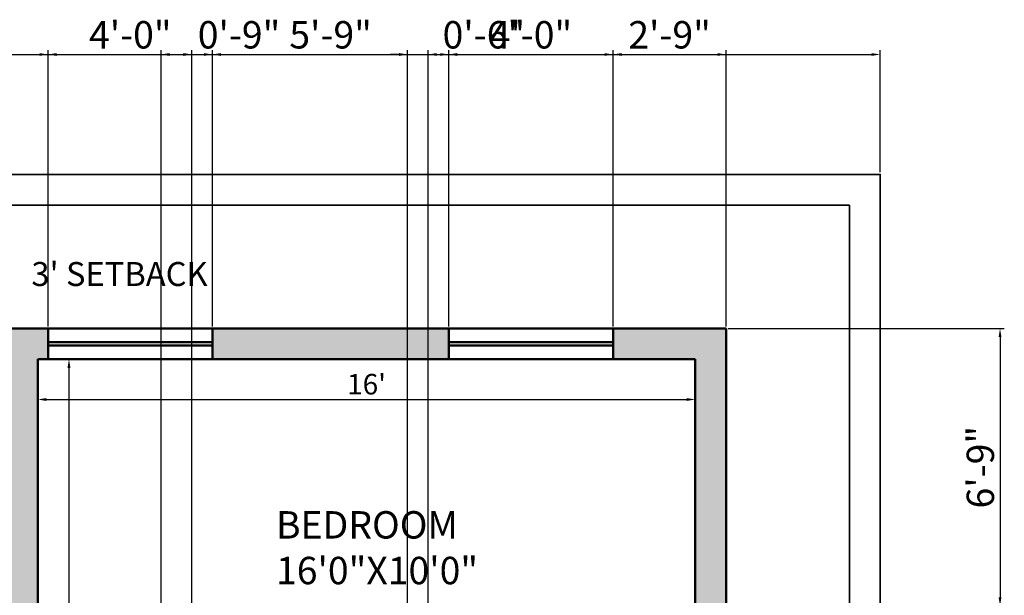
# Model space of a CAD drawing. Units: inches. Extents: x 2442 to 3851, y 589 to 2836.
# Tile 22 of 22: x 3558 to 3845, y 2668 to 2836. Entities that reach past the tile are written whole.
import ezdxf

# ---------------------------------------------------------------- set-up
doc = ezdxf.new("R2010")
doc.units = ezdxf.units.IN
for name, color, linetype, lineweight in [('A-ANNO-DIMS', 2, 'Continuous', 18), ('A-ANNO-TEXT', 7, 'Continuous', 18), ('A-AREA-IDEN', 7, 'Continuous', 18), ('A-WALL', 7, 'Continuous', 50), ('A-WALL-PATT', 8, 'Continuous', 13), ('C-PROP', 7, 'Continuous', 35)]:
    doc.layers.add(name, color=color, linetype=linetype, lineweight=lineweight)
doc.styles.get("Standard").update_dxf_attribs({"font": 'arial.ttf'})
doc.dimstyles.new('ISO-25', dxfattribs={"dimtxt": 8, "dimasz": 2.5, "dimexe": 1.25, "dimexo": 0.625, "dimtad": 1, "dimlunit": 3, "dimtxsty": 'Standard', "dimcen": 2.5, "dimadec": 0, "dimazin": 0, "dimtfac": 1, "dimtmove": 0, "dimatfit": 3, "dimfxl": 1, "dimarcsym": 0})

# ---------------------------------------------------------------- blocks, each defined once
blk = doc.blocks.new('*D116')
at = {"layer": 'A-ANNO-DIMS', "color": 0, "lineweight": -2, "transparency": 16777216}
for p, q in [((3563.02, 2736.58), (3563.02, 2724.22)), ((3755.02, 2736.58), (3755.02, 2724.22)), ((3565.52, 2725.47), (3752.52, 2725.47))]:
    blk.add_line(p, q, dxfattribs=at)
at = {"layer": 'A-ANNO-DIMS', "color": 0, "transparency": 16777216}
for points in [[(3565.52, 2725.89), (3565.52, 2725.05), (3563.02, 2725.47)], [(3752.52, 2725.89), (3752.52, 2725.05), (3755.02, 2725.47)]]:
    blk.add_solid(points, dxfattribs=at)
at = {"layer": 'Defpoints', "color": 0, "transparency": 16777216}
for p in [(3563.02, 2737.21), (3755.02, 2737.21), (3755.02, 2725.47)]:
    blk.add_point(p, dxfattribs=at)
at = {"layer": 'A-ANNO-DIMS', "color": 0, "transparency": 16777216, "insert": (3659.02, 2729.16), "char_height": 6, "attachment_point": 5}
blk.add_mtext("16'", dxfattribs=at)
blk = doc.blocks.new('*D117')
at = {"layer": 'A-ANNO-DIMS', "color": 0, "lineweight": -2, "transparency": 16777216}
for p, q in [((3563.65, 2737.21), (3573.36, 2737.21)), ((3572.11, 2734.71), (3572.11, 2565.71)), ((3563.65, 2563.21), (3573.36, 2563.21))]:
    blk.add_line(p, q, dxfattribs=at)
at = {"layer": 'A-ANNO-DIMS', "color": 0, "transparency": 16777216}
for points in [[(3571.69, 2734.71), (3572.53, 2734.71), (3572.11, 2737.21)], [(3571.69, 2565.71), (3572.53, 2565.71), (3572.11, 2563.21)]]:
    blk.add_solid(points, dxfattribs=at)
at = {"layer": 'Defpoints', "color": 0, "transparency": 16777216}
for p in [(3563.02, 2737.21), (3563.02, 2563.21), (3572.11, 2563.21)]:
    blk.add_point(p, dxfattribs=at)
at = {"layer": 'A-ANNO-DIMS', "color": 0, "transparency": 16777216, "insert": (3568.42, 2650.21), "char_height": 6, "attachment_point": 5, "rotation": 90}
blk.add_mtext('14\'-6"', dxfattribs=at)
blk = doc.blocks.new('*D218')
at = {"layer": 'A-ANNO-DIMS', "color": 0, "lineweight": -2, "transparency": 16777216}
for p, q in [((3209.02, 2791.83), (3209.02, 2827.46)), ((3809.02, 2791.83), (3809.02, 2827.46)), ((3211.52, 2826.21), (3806.52, 2826.21))]:
    blk.add_line(p, q, dxfattribs=at)
at = {"layer": 'A-ANNO-DIMS', "color": 0, "transparency": 16777216}
for points in [[(3211.52, 2826.62), (3211.52, 2825.79), (3209.02, 2826.21)], [(3806.52, 2826.62), (3806.52, 2825.79), (3809.02, 2826.21)]]:
    blk.add_solid(points, dxfattribs=at)
at = {"layer": 'Defpoints', "color": 0, "transparency": 16777216}
for p in [(3809.02, 2826.21), (3209.02, 2791.21), (3809.02, 2791.21)]:
    blk.add_point(p, dxfattribs=at)
at = {"layer": 'A-ANNO-DIMS', "color": 0, "transparency": 16777216, "insert": (3509.02, 2830.92), "char_height": 8, "attachment_point": 5}
blk.add_mtext('50\'-0"', dxfattribs=at)
blk = doc.blocks.new('*D222')
at = {"layer": 'A-ANNO-DIMS', "color": 0, "lineweight": -2, "transparency": 16777216}
for p, q in [((3512.02, 2746.83), (3512.02, 2827.46)), ((3566.02, 2746.83), (3566.02, 2827.46)), ((3514.52, 2826.21), (3563.52, 2826.21))]:
    blk.add_line(p, q, dxfattribs=at)
at = {"layer": 'A-ANNO-DIMS', "color": 0, "transparency": 16777216}
for points in [[(3514.52, 2826.62), (3514.52, 2825.79), (3512.02, 2826.21)], [(3563.52, 2826.62), (3563.52, 2825.79), (3566.02, 2826.21)]]:
    blk.add_solid(points, dxfattribs=at)
at = {"layer": 'Defpoints', "color": 0, "transparency": 16777216}
for p in [(3566.02, 2826.21), (3512.02, 2746.21), (3566.02, 2746.21)]:
    blk.add_point(p, dxfattribs=at)
at = {"layer": 'A-ANNO-DIMS', "color": 0, "transparency": 16777216, "insert": (3539.02, 2830.92), "char_height": 8, "attachment_point": 5}
blk.add_mtext('4\'-6"', dxfattribs=at)
blk = doc.blocks.new('*D223')
at = {"layer": 'A-ANNO-DIMS', "color": 0, "lineweight": -2, "transparency": 16777216}
for p, q in [((3566.02, 2746.83), (3566.02, 2827.46)), ((3614.02, 2746.83), (3614.02, 2827.46)), ((3568.52, 2826.21), (3611.52, 2826.21))]:
    blk.add_line(p, q, dxfattribs=at)
at = {"layer": 'A-ANNO-DIMS', "color": 0, "transparency": 16777216}
for points in [[(3568.52, 2826.62), (3568.52, 2825.79), (3566.02, 2826.21)], [(3611.52, 2826.62), (3611.52, 2825.79), (3614.02, 2826.21)]]:
    blk.add_solid(points, dxfattribs=at)
at = {"layer": 'Defpoints', "color": 0, "transparency": 16777216}
for p in [(3614.02, 2826.21), (3566.02, 2746.21), (3614.02, 2746.21)]:
    blk.add_point(p, dxfattribs=at)
at = {"layer": 'A-ANNO-DIMS', "color": 0, "transparency": 16777216, "insert": (3590.02, 2830.92), "char_height": 8, "attachment_point": 5}
blk.add_mtext('4\'-0"', dxfattribs=at)
blk = doc.blocks.new('*D224')
at = {"layer": 'A-ANNO-DIMS', "color": 0, "lineweight": -2, "transparency": 16777216}
for p, q in [((3614.02, 2746.83), (3614.02, 2827.46)), ((3683.02, 2746.83), (3683.02, 2827.46)), ((3616.52, 2826.21), (3680.52, 2826.21))]:
    blk.add_line(p, q, dxfattribs=at)
at = {"layer": 'A-ANNO-DIMS', "color": 0, "transparency": 16777216}
for points in [[(3616.52, 2826.62), (3616.52, 2825.79), (3614.02, 2826.21)], [(3680.52, 2826.62), (3680.52, 2825.79), (3683.02, 2826.21)]]:
    blk.add_solid(points, dxfattribs=at)
at = {"layer": 'Defpoints', "color": 0, "transparency": 16777216}
for p in [(3683.02, 2826.21), (3614.02, 2746.21), (3683.02, 2746.21)]:
    blk.add_point(p, dxfattribs=at)
at = {"layer": 'A-ANNO-DIMS', "color": 0, "transparency": 16777216, "insert": (3648.52, 2830.92), "char_height": 8, "attachment_point": 5}
blk.add_mtext('5\'-9"', dxfattribs=at)
blk = doc.blocks.new('*D225')
at = {"layer": 'A-ANNO-DIMS', "color": 0, "lineweight": -2, "transparency": 16777216}
for p, q in [((3683.02, 2746.83), (3683.02, 2827.46)), ((3731.02, 2746.83), (3731.02, 2827.46)), ((3685.52, 2826.21), (3728.52, 2826.21))]:
    blk.add_line(p, q, dxfattribs=at)
at = {"layer": 'A-ANNO-DIMS', "color": 0, "transparency": 16777216}
for points in [[(3685.52, 2826.62), (3685.52, 2825.79), (3683.02, 2826.21)], [(3728.52, 2826.62), (3728.52, 2825.79), (3731.02, 2826.21)]]:
    blk.add_solid(points, dxfattribs=at)
at = {"layer": 'Defpoints', "color": 0, "transparency": 16777216}
for p in [(3731.02, 2826.21), (3683.02, 2746.21), (3731.02, 2746.21)]:
    blk.add_point(p, dxfattribs=at)
at = {"layer": 'A-ANNO-DIMS', "color": 0, "transparency": 16777216, "insert": (3707.02, 2830.92), "char_height": 8, "attachment_point": 5}
blk.add_mtext('4\'-0"', dxfattribs=at)
blk = doc.blocks.new('*D226')
at = {"layer": 'A-ANNO-DIMS', "color": 0, "lineweight": -2, "transparency": 16777216}
for p, q in [((3731.02, 2746.83), (3731.02, 2827.46)), ((3764.02, 2746.83), (3764.02, 2827.46)), ((3733.52, 2826.21), (3761.52, 2826.21))]:
    blk.add_line(p, q, dxfattribs=at)
at = {"layer": 'A-ANNO-DIMS', "color": 0, "transparency": 16777216}
for points in [[(3733.52, 2826.62), (3733.52, 2825.79), (3731.02, 2826.21)], [(3761.52, 2826.62), (3761.52, 2825.79), (3764.02, 2826.21)]]:
    blk.add_solid(points, dxfattribs=at)
at = {"layer": 'Defpoints', "color": 0, "transparency": 16777216}
for p in [(3764.02, 2826.21), (3731.02, 2746.21), (3764.02, 2746.21)]:
    blk.add_point(p, dxfattribs=at)
at = {"layer": 'A-ANNO-DIMS', "color": 0, "transparency": 16777216, "insert": (3747.52, 2830.92), "char_height": 8, "attachment_point": 5}
blk.add_mtext('2\'-9"', dxfattribs=at)
blk = doc.blocks.new('*D227')
at = {"layer": 'A-ANNO-DIMS', "color": 0, "lineweight": -2, "transparency": 16777216}
for p, q in [((3764.65, 2746.21), (3845.27, 2746.21)), ((3844.02, 2743.71), (3844.02, 2667.71)), ((3764.65, 2665.21), (3845.27, 2665.21))]:
    blk.add_line(p, q, dxfattribs=at)
at = {"layer": 'A-ANNO-DIMS', "color": 0, "transparency": 16777216}
for points in [[(3843.61, 2743.71), (3844.44, 2743.71), (3844.02, 2746.21)], [(3843.61, 2667.71), (3844.44, 2667.71), (3844.02, 2665.21)]]:
    blk.add_solid(points, dxfattribs=at)
at = {"layer": 'Defpoints', "color": 0, "transparency": 16777216}
for p in [(3764.02, 2746.21), (3764.02, 2665.21), (3844.02, 2665.21)]:
    blk.add_point(p, dxfattribs=at)
at = {"layer": 'A-ANNO-DIMS', "color": 0, "transparency": 16777216, "insert": (3839.31, 2705.71), "char_height": 8, "attachment_point": 5, "rotation": 90}
blk.add_mtext('6\'-9"', dxfattribs=at)
blk = doc.blocks.new('*D253')
at = {"layer": 'A-ANNO-DIMS', "color": 0, "lineweight": -2, "transparency": 16777216}
for p, q in [((3599.02, 2461.83), (3599.02, 2827.46)), ((3608.02, 2461.83), (3608.02, 2827.46)), ((3601.52, 2826.21), (3605.52, 2826.21)), ((3608.02, 2826.21), (3633.04, 2826.21))]:
    blk.add_line(p, q, dxfattribs=at)
at = {"layer": 'A-ANNO-DIMS', "color": 0, "transparency": 16777216}
for points in [[(3601.52, 2826.62), (3601.52, 2825.79), (3599.02, 2826.21)], [(3605.52, 2826.62), (3605.52, 2825.79), (3608.02, 2826.21)]]:
    blk.add_solid(points, dxfattribs=at)
at = {"layer": 'Defpoints', "color": 0, "transparency": 16777216}
for p in [(3608.02, 2826.21), (3599.02, 2461.21), (3608.02, 2461.21)]:
    blk.add_point(p, dxfattribs=at)
at = {"layer": 'A-ANNO-DIMS', "color": 0, "transparency": 16777216, "insert": (3621.78, 2830.92), "char_height": 8, "attachment_point": 5}
blk.add_mtext('0\'-9"', dxfattribs=at)
blk = doc.blocks.new('*D254')
at = {"layer": 'A-ANNO-DIMS', "color": 0, "lineweight": -2, "transparency": 16777216}
for p, q in [((3671.02, 2581.83), (3671.02, 2827.46)), ((3677.02, 2581.83), (3677.02, 2827.46)), ((3668.52, 2826.21), (3666.02, 2826.21)), ((3671.02, 2826.21), (3677.02, 2826.21)), ((3679.52, 2826.21), (3704.54, 2826.21))]:
    blk.add_line(p, q, dxfattribs=at)
at = {"layer": 'A-ANNO-DIMS', "color": 0, "transparency": 16777216}
for points in [[(3668.52, 2826.62), (3668.52, 2825.79), (3671.02, 2826.21)], [(3679.52, 2826.62), (3679.52, 2825.79), (3677.02, 2826.21)]]:
    blk.add_solid(points, dxfattribs=at)
at = {"layer": 'Defpoints', "color": 0, "transparency": 16777216}
for p in [(3677.02, 2826.21), (3671.02, 2581.21), (3677.02, 2581.21)]:
    blk.add_point(p, dxfattribs=at)
at = {"layer": 'A-ANNO-DIMS', "color": 0, "transparency": 16777216, "insert": (3693.28, 2830.92), "char_height": 8, "attachment_point": 5}
blk.add_mtext('0\'-6"', dxfattribs=at)

msp = doc.modelspace()

# ---------------------------------------------------------------- hatches: boundary and pattern name
at = {"layer": 'A-WALL-PATT'}
h = msp.add_hatch(color=256, dxfattribs=at)
h.dxf.hatch_style = 1
h.paths.add_polyline_path([(3356.024, 2713.208), (3356.024, 2719.208), (3356.024, 2722.208), (3254.024, 2722.208), (3254.024, 2657.708), (3263.024, 2657.708), (3263.024, 2713.208)])
h.paths.add_polyline_path([(3416.024, 2737.208), (3446.024, 2737.208), (3446.024, 2746.208), (3416.024, 2746.208), (3416.024, 2782.208), (3407.024, 2782.208), (3407.024, 2722.208), (3386.024, 2722.208), (3386.024, 2719.208), (3386.024, 2713.208), (3407.024, 2713.208), (3407.024, 2593.208), (3416.024, 2593.208), (3416.024, 2608.208), (3515.024, 2608.208), (3515.024, 2614.208), (3515.024, 2617.208), (3416.024, 2617.208)])
h.paths.add_polyline_path([(3563.024, 2737.208), (3566.024, 2737.208), (3566.024, 2746.208), (3512.024, 2746.208), (3512.024, 2737.208), (3554.024, 2737.208), (3554.024, 2617.208), (3551.024, 2617.208), (3551.024, 2614.208), (3551.024, 2608.208), (3554.024, 2608.208), (3554.024, 2554.208), (3566.024, 2554.208), (3566.024, 2560.208), (3566.024, 2563.208), (3563.024, 2563.208)])
h.paths.add_polyline_path([(3614.024, 2746.208), (3614.024, 2737.208), (3683.024, 2737.208), (3683.024, 2746.208)])
h.paths.add_polyline_path([(3755.024, 2737.208), (3755.024, 2665.208), (3764.024, 2665.208), (3764.024, 2746.208), (3731.024, 2746.208), (3731.024, 2737.208)])
h.paths.add_polyline_path([(3662.024, 2617.208), (3662.024, 2611.208), (3755.024, 2611.208), (3755.024, 2605.208), (3764.024, 2605.208), (3764.024, 2617.208)])
h.paths.add_polyline_path([(3755.024, 2554.208), (3755.024, 2548.208), (3764.024, 2548.208), (3764.024, 2569.208), (3755.024, 2569.208), (3755.024, 2563.208), (3677.024, 2563.208), (3677.024, 2581.208), (3671.024, 2581.208), (3671.024, 2563.208), (3611.024, 2563.208), (3611.024, 2611.208), (3632.024, 2611.208), (3632.024, 2617.208), (3605.024, 2617.208), (3605.024, 2563.208), (3602.024, 2563.208), (3602.024, 2554.208), (3653.024, 2554.208), (3653.024, 2536.208), (3659.024, 2536.208), (3659.024, 2554.208)])
h.paths.add_polyline_path([(3764.024, 2512.208), (3755.024, 2512.208), (3755.024, 2506.208), (3653.024, 2506.208), (3653.024, 2500.208), (3755.024, 2500.208), (3755.024, 2474.708), (3764.024, 2474.708)])
h.paths.add_polyline_path([(3608.024, 2392.208), (3764.024, 2392.208), (3764.024, 2426.708), (3755.024, 2426.708), (3755.024, 2401.208), (3608.024, 2401.208), (3608.024, 2461.208), (3599.024, 2461.208), (3599.024, 2353.208), (3608.024, 2353.208)])
h.paths.add_polyline_path([(3410.024, 2401.208), (3263.024, 2401.208), (3263.024, 2473.208), (3254.024, 2473.208), (3254.024, 2368.208), (3263.024, 2368.208), (3263.024, 2392.208), (3410.024, 2392.208), (3410.024, 2344.208), (3419.024, 2344.208), (3419.024, 2506.208), (3413.024, 2506.208), (3410.024, 2506.208)])
h.paths.add_polyline_path([(3263.024, 2609.708), (3254.024, 2609.708), (3254.024, 2521.208), (3263.024, 2521.208), (3263.024, 2545.208), (3410.024, 2545.208), (3410.024, 2542.208), (3413.024, 2542.208), (3419.024, 2542.208), (3419.024, 2557.208), (3407.024, 2557.208), (3407.024, 2554.208), (3263.024, 2554.208)])
h.paths.add_polyline_path([(3254.024, 2191.208), (3263.024, 2191.208), (3263.024, 2287.208), (3269.024, 2287.208), (3269.024, 2293.208), (3269.024, 2296.208), (3263.024, 2296.208), (3263.024, 2320.208), (3254.024, 2320.208)])
h.paths.add_polyline_path([(3419.024, 2296.208), (3386.024, 2296.208), (3386.024, 2287.208), (3410.024, 2287.208), (3410.024, 2191.208), (3419.024, 2191.208), (3419.024, 2248.208), (3449.024, 2248.208), (3449.024, 2257.208), (3419.024, 2257.208)])
h.paths.add_polyline_path([(3581.024, 2248.208), (3608.024, 2248.208), (3608.024, 2287.208), (3599.024, 2287.208), (3599.024, 2257.208), (3581.024, 2257.208)])
h.paths.add_polyline_path([(3491.024, 2248.208), (3515.024, 2248.208), (3515.024, 2257.208), (3491.024, 2257.208)])
h.paths.add_polyline_path([(3320.024, 2296.208), (3309.024, 2296.208), (3309.024, 2287.208), (3320.024, 2287.208)])
h.paths.add_polyline_path([(3282.007, 2631.263), (3387.059, 2631.263), (3387.059, 2661.678), (3282.007, 2661.678)], flags=9)
h.paths.add_polyline_path([(3511.253, 2214.916), (3571.545, 2214.916), (3571.545, 2229.862), (3511.253, 2229.862)], flags=9)
h.paths.add_polyline_path([(3777.335, 2589.915), (3777.335, 2529.623), (3792.281, 2529.623), (3792.281, 2589.915)], flags=9)
h.paths.add_polyline_path([(3558.97, 2754.629), (3619.262, 2754.629), (3619.262, 2769.575), (3558.97, 2769.575)], flags=9)
h.paths.add_polyline_path([(3314.979, 2749.318), (3377.263, 2749.318), (3377.263, 2779.733), (3314.979, 2779.733)], flags=9)
h.paths.add_polyline_path([(3624.453, 2577.252), (3671.045, 2577.252), (3671.045, 2600.063), (3624.453, 2600.063)], flags=25)
h.paths.add_polyline_path([(3701.15, 2577.252), (3744.07, 2577.252), (3744.07, 2600.063), (3701.15, 2600.063)], flags=25)
h.paths.add_polyline_path([(3689.533, 2518.545), (3731.868, 2518.545), (3731.868, 2541.356), (3689.533, 2541.356)], flags=9)
h.paths.add_polyline_path([(3629.196, 2666.979), (3693.452, 2666.979), (3693.452, 2697.394), (3629.196, 2697.394)], flags=9)
h.paths.add_polyline_path([(3441.284, 2669.891), (3505.54, 2669.891), (3505.54, 2700.306), (3441.284, 2700.306)], flags=25)
h.paths.add_polyline_path([(3306.565, 2459.233), (3370.821, 2459.233), (3370.821, 2489.648), (3306.565, 2489.648)], flags=25)
h.paths.add_polyline_path([(3307.889, 2320.733), (3387.355, 2320.733), (3387.355, 2351.148), (3307.889, 2351.148)], flags=9)
h.paths.add_polyline_path([(3452.987, 2372.794), (3554.971, 2372.794), (3554.971, 2403.208), (3452.987, 2403.208)], flags=9)

# ---------------------------------------------------------------- linework, layer by layer
at = {"layer": 'A-WALL'}
for p, q in [((3416.024, 2746.208), (3764.024, 2746.208)), ((3566.024, 2737.208), (3566.024, 2746.208)), ((3614.024, 2737.208), (3614.024, 2746.208)), ((3683.024, 2737.208), (3683.024, 2746.208)), ((3731.024, 2737.208), (3731.024, 2746.208)), ((3764.024, 2392.208), (3764.024, 2746.208)), ((3566.024, 2742.208), (3614.024, 2742.208)), ((3566.024, 2741.208), (3614.024, 2741.208)), ((3683.024, 2742.208), (3731.024, 2742.208)), ((3683.024, 2741.208), (3731.024, 2741.208)), ((3563.024, 2563.208), (3563.024, 2737.208)), ((3563.024, 2737.208), (3755.024, 2737.208)), ((3755.024, 2617.208), (3755.024, 2737.208))]:
    msp.add_line(p, q, dxfattribs=at)
at = {"layer": 'C-PROP'}
for points in [[(3809.024, 2191.208), (3809.024, 2791.208), (3209.024, 2791.208), (3209.024, 2191.208), (3809.024, 2191.208)], [(3800.024, 2200.208), (3800.024, 2782.208), (3218.024, 2782.208), (3218.024, 2200.208), (3254.024, 2200.208)]]:
    msp.add_lwpolyline(points, dxfattribs=at)

# ---------------------------------------------------------------- texts
at = {"layer": 'A-ANNO-TEXT', "insert": (3561.139, 2765.614), "char_height": 7, "attachment_point": 1}
msp.add_mtext_dynamic_manual_height_columns("{\\fTimes New Roman|b0|i0|c0|p18;3' SETBACK}", width=79.56037, gutter_width=12.5, heights=[0], dxfattribs=at)
at = {"layer": 'A-AREA-IDEN', "insert": (3632.58, 2692.868), "char_height": 8, "attachment_point": 1}
msp.add_mtext_dynamic_manual_height_columns('{\\fTimes New Roman|b0|i0|c0|p18;BEDROOM\\P16\'0"X10\'0"}', width=110.76054, gutter_width=12.5, heights=[0], dxfattribs=at)

# ---------------------------------------------------------------- dimensions: what is measured, and where the dimension line sits
at = {"layer": 'A-ANNO-DIMS'}
for base, p1, p2, override, picture, middle in [((3809.024, 2826.208), (3209.024, 2791.208), (3809.024, 2791.208), {"dimdec": 1, "dimlfac": 1, "dimrnd": 0, "dimzin": 1, "dimdsep": 46, "dimlunit": 4, "dimfrac": 2}, '*D218', (3509.024, 2830.917)), ((3566.024, 2826.208), (3512.024, 2746.208), (3566.024, 2746.208), {"dimdec": 1, "dimlfac": 1, "dimrnd": 0, "dimzin": 1, "dimdsep": 46, "dimlunit": 4, "dimfrac": 2}, '*D222', (3539.024, 2830.917)), ((3614.024, 2826.208), (3566.024, 2746.208), (3614.024, 2746.208), {"dimdec": 1, "dimlfac": 1, "dimrnd": 0, "dimzin": 1, "dimdsep": 46, "dimlunit": 4, "dimfrac": 2}, '*D223', (3590.024, 2830.917)), ((3608.024, 2826.208), (3599.024, 2461.208), (3608.024, 2461.208), {"dimdec": 1, "dimlfac": 1, "dimrnd": 0, "dimzin": 1, "dimdsep": 46, "dimlunit": 4, "dimfrac": 2}, '*D253', (3621.783, 2830.917)), ((3683.024, 2826.208), (3614.024, 2746.208), (3683.024, 2746.208), {"dimdec": 1, "dimlfac": 1, "dimrnd": 0, "dimzin": 1, "dimdsep": 46, "dimlunit": 4, "dimfrac": 2}, '*D224', (3648.524, 2830.917)), ((3677.024, 2826.208), (3671.024, 2581.208), (3677.024, 2581.208), {"dimdec": 1, "dimlfac": 1, "dimrnd": 0, "dimzin": 1, "dimdsep": 46, "dimlunit": 4, "dimfrac": 2}, '*D254', (3693.283, 2830.917)), ((3731.024, 2826.208), (3683.024, 2746.208), (3731.024, 2746.208), {"dimdec": 1, "dimlfac": 1, "dimrnd": 0, "dimzin": 1, "dimdsep": 46, "dimlunit": 4, "dimfrac": 2}, '*D225', (3707.024, 2830.917)), ((3764.024, 2826.208), (3731.024, 2746.208), (3764.024, 2746.208), {"dimdec": 1, "dimlfac": 1, "dimrnd": 0, "dimzin": 1, "dimdsep": 46, "dimlunit": 4, "dimfrac": 2}, '*D226', (3747.524, 2830.917)), ((3755.024, 2725.472), (3563.024, 2737.208), (3755.024, 2737.208), {"dimtxt": 6, "dimclrd": 0, "dimclre": 0, "dimclrt": 0}, '*D116', (3659.024, 2729.16))]:
    dim = msp.add_linear_dim(base=base, p1=p1, p2=p2, dimstyle='ISO-25', override=override, dxfattribs=at)
    dim.commit()
    dim.dimension.update_dxf_attribs({"geometry": picture, "text_midpoint": middle})
for base, p1, p2, override, picture, middle in [((3844.024, 2665.208), (3764.024, 2746.208), (3764.024, 2665.208), {"dimdec": 1, "dimlfac": 1, "dimrnd": 0, "dimzin": 1, "dimdsep": 46, "dimlunit": 4, "dimfrac": 2}, '*D227', (3839.315, 2705.708)), ((3572.11, 2563.208), (3563.024, 2737.208), (3563.024, 2563.208), {"dimtxt": 6, "dimclrd": 0, "dimclre": 0, "dimclrt": 0}, '*D117', (3568.422, 2650.208))]:
    dim = msp.add_linear_dim(base=base, p1=p1, p2=p2, angle=90, dimstyle='ISO-25', override=override, dxfattribs=at)
    dim.commit()
    dim.dimension.update_dxf_attribs({"geometry": picture, "text_midpoint": middle})

doc.saveas('drawing.dxf')
